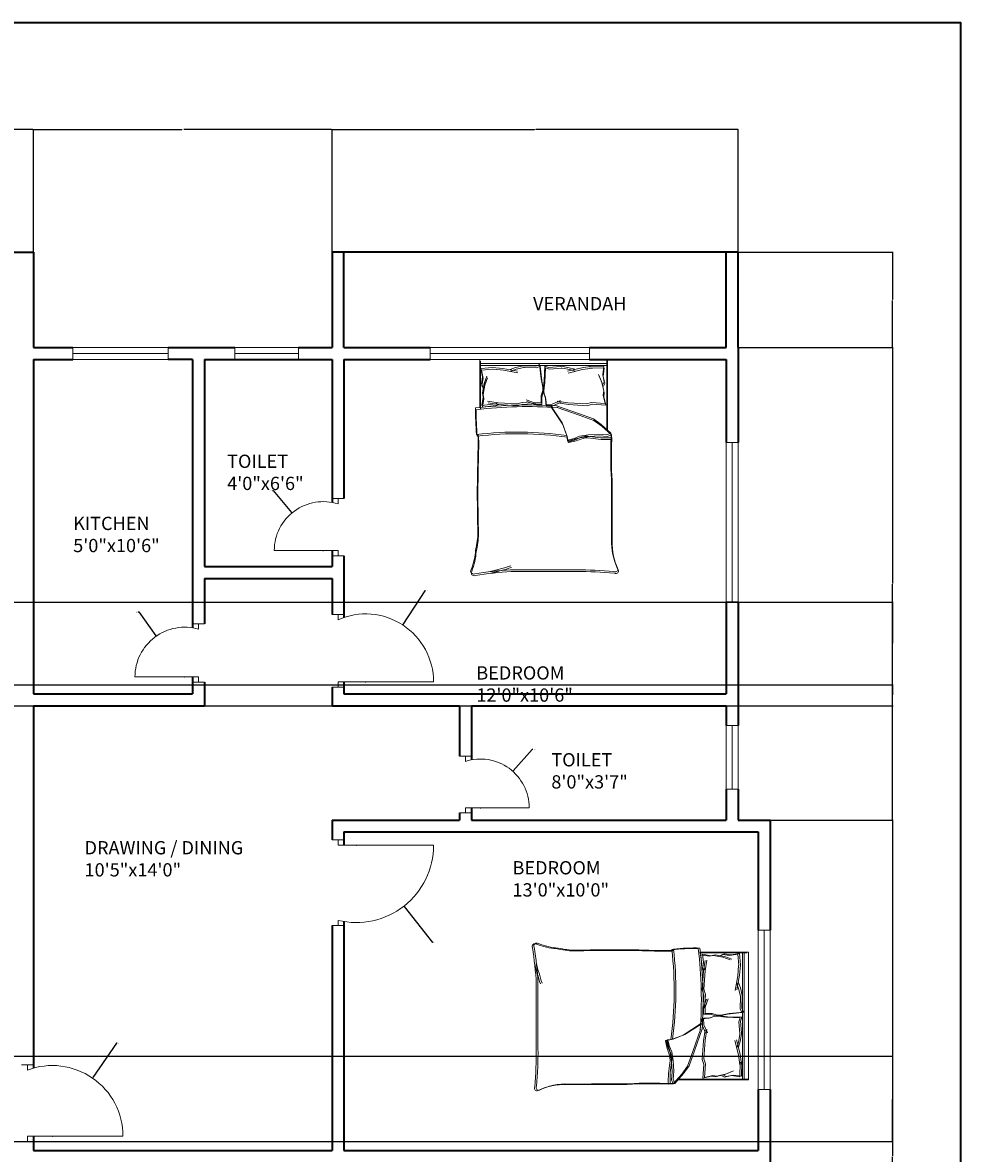
# Model space of a CAD drawing. Units: inches. Extents: x 1937 to 2996, y 1402 to 2323.
# Tile 10 of 10: x 2643 to 2996, y 1897 to 2323. Entities that reach past the tile are written whole.
import ezdxf

# ---------------------------------------------------------------- set-up
doc = ezdxf.new("R2010")
doc.units = ezdxf.units.IN
for name, color, linetype, lineweight in [('A-ANNO-DIMS', 2, 'Continuous', 18), ('A-ANNO-TTLB', 7, 'Continuous', 35), ('A-AREA-IDEN', 7, 'Continuous', 18), ('A-DOOR', 11, 'Continuous', 18), ('A-FURN', 8, 'Continuous', 13), ('A-GLAZ', 141, 'Continuous', 18), ('A-WALL', 7, 'Continuous', 35)]:
    doc.layers.add(name, color=color, linetype=linetype, lineweight=lineweight)
doc.styles.get("Standard").update_dxf_attribs({"font": 'arial.ttf'})
doc.dimstyles.get("Standard").update_dxf_attribs({"dimtxt": 0.18, "dimasz": 0.18, "dimexe": 0.18, "dimexo": 0.0625, "dimgap": 0.09, "dimtad": 0, "dimtih": 1, "dimtoh": 1, "dimdec": 4, "dimzin": 0, "dimdsep": 46, "dimtxsty": 'Standard', "dimcen": 0.09, "dimadec": 0, "dimazin": 0, "dimtfac": 1, "dimtdec": 4, "dimtofl": 0, "dimtmove": 0, "dimatfit": 3, "dimfxl": 1, "dimtolj": 1, "dimtzin": 0, "dimarcsym": 0})

# ---------------------------------------------------------------- blocks, each defined once
blk = doc.blocks.new('BED-DOUBLE')
for p, q in [((-24.01, -18.11), (-24.01, 0)), ((-24.01, -18.11), (-24.01, 0)), ((-24.01, 0), (24.01, 0)), ((23.78, 0), (23.78, -26.61)), ((23.78, 0), (23.78, -26.61)), ((24.01, 0), (24.01, -0.64)), ((-24.01, -1.53), (23.78, -1.53)), ((-24.01, -1.53), (23.78, -1.53)), ((-23.78, -18.75), (-23.78, -0.64)), ((-23.78, -18.75), (-23.78, -0.64)), ((-23.78, -2.17), (24.01, -2.17)), ((-23.78, -2.17), (24.01, -2.17)), ((-23.59, -3.34), (-19.3, -3.01)), ((-23.59, -3.34), (-19.31, -3.01)), ((-23.59, -3.32), (-23.01, -6.5)), ((-23.59, -3.32), (-23.01, -6.5)), ((-23.36, -3.98), (-19.08, -3.65)), ((-23.36, -3.98), (-19.08, -3.65)), ((-23.36, -3.96), (-22.78, -7.14)), ((-23.36, -3.96), (-22.78, -7.14)), ((-19.31, -3.01), (-19.2, -3.03)), ((-19.3, -3.01), (-19.2, -3.03)), ((-19.2, -3.03), (-15.38, -3.32)), ((-19.2, -3.03), (-15.38, -3.32)), ((-19.08, -3.65), (-18.97, -3.67)), ((-19.08, -3.65), (-18.97, -3.67)), ((-18.97, -3.67), (-15.15, -3.96)), ((-18.97, -3.67), (-15.15, -3.96)), ((-15.38, -3.32), (-9.88, -4.33)), ((-15.38, -3.32), (-9.88, -4.33)), ((-15.15, -3.96), (-9.65, -4.97)), ((-15.15, -3.96), (-9.65, -4.97)), ((-12.63, -3.75), (-10.61, -3.03)), ((-12.63, -3.75), (-10.61, -3.03)), ((-12.4, -4.39), (-10.38, -3.67)), ((-12.4, -4.39), (-10.38, -3.67)), ((-10.61, -3.03), (-7.71, -2.3)), ((-10.61, -3.03), (-7.71, -2.3)), ((-10.38, -3.67), (-7.49, -2.94)), ((-10.38, -3.67), (-7.49, -2.94)), ((-7.71, -2.3), (-7.39, -2.3)), ((-7.71, -2.3), (-7.39, -2.3)), ((-7.49, -2.94), (-7.16, -2.94)), ((-7.49, -2.94), (-7.16, -2.94)), ((-7.39, -2.3), (-2.95, -2.45)), ((-7.39, -2.3), (-2.95, -2.45)), ((-7.16, -2.94), (-2.72, -3.09)), ((-7.16, -2.94), (-2.72, -3.09)), ((-2.95, -2.45), (-1.5, -1.87)), ((-2.95, -2.45), (-1.5, -1.87)), ((-2.72, -3.09), (-1.27, -2.51)), ((-2.72, -3.09), (-1.27, -2.51)), ((-1.5, -1.87), (-0.92, -7.22)), ((-1.5, -1.87), (-0.92, -7.22)), ((-1.27, -2.51), (-0.7, -7.86)), ((-1.27, -2.51), (-0.7, -7.86)), ((0.49, -2.49), (0.25, -7.87)), ((0.49, -2.49), (0.25, -7.87)), ((0.72, -3.13), (0.48, -8.51)), ((0.72, -3.13), (0.48, -8.51)), ((1.97, -2.98), (0.49, -2.49)), ((1.97, -2.98), (0.49, -2.49)), ((2.2, -3.62), (0.72, -3.13)), ((2.2, -3.62), (0.72, -3.13)), ((6.4, -2.56), (1.97, -2.98)), ((6.4, -2.56), (1.97, -2.98)), ((6.63, -3.2), (2.2, -3.62)), ((6.63, -3.2), (2.2, -3.62)), ((6.72, -2.54), (6.4, -2.56)), ((6.72, -2.54), (6.4, -2.56)), ((6.95, -3.18), (6.63, -3.2)), ((6.95, -3.18), (6.63, -3.2)), ((9.65, -3.08), (6.72, -2.54)), ((9.65, -3.08), (6.72, -2.54)), ((9.88, -3.72), (6.95, -3.18)), ((9.88, -3.72), (6.95, -3.18)), ((14.43, -3.07), (9.01, -4.42)), ((14.43, -3.07), (9.01, -4.42)), ((14.66, -3.71), (9.24, -5.06)), ((14.66, -3.71), (9.24, -5.06)), ((11.72, -3.67), (9.65, -3.08)), ((11.72, -3.67), (9.65, -3.08)), ((11.94, -4.31), (9.88, -3.72)), ((11.94, -4.31), (9.88, -3.72)), ((18.23, -2.54), (14.43, -3.07)), ((18.23, -2.54), (14.43, -3.07)), ((18.46, -3.18), (14.66, -3.71)), ((18.46, -3.18), (14.66, -3.71)), ((22.63, -2.56), (17.23, -2.46)), ((17.23, -2.46), (18.23, -2.54)), ((22.63, -2.56), (17.23, -2.46)), ((17.23, -2.46), (18.23, -2.54)), ((22.86, -3.2), (17.45, -3.1)), ((17.45, -3.1), (18.46, -3.18)), ((22.86, -3.2), (17.45, -3.1)), ((17.45, -3.1), (18.46, -3.18)), ((22.63, -2.56), (22.25, -5.77)), ((22.63, -2.56), (22.25, -5.77)), ((22.86, -3.2), (22.48, -6.41)), ((22.86, -3.2), (22.48, -6.41)), ((24.01, -0.64), (24.01, -27.25)), ((24.01, -0.64), (24.01, -27.25)), ((-23.01, -6.5), (-23.45, -9.1)), ((-23.01, -6.5), (-23.45, -9.1)), ((-22.78, -7.14), (-23.22, -9.74)), ((-22.78, -7.14), (-23.22, -9.74)), ((-22.43, -8.96), (-21.42, -6.21)), ((-22.43, -8.96), (-21.42, -6.21)), ((-22.21, -9.59), (-21.19, -6.85)), ((-22.2, -9.59), (-21.19, -6.85)), ((-0.92, -7.22), (-0.35, -10.4)), ((-0.92, -7.22), (-0.35, -10.4)), ((-0.7, -7.86), (-0.12, -11.04)), ((-0.7, -7.86), (-0.12, -11.04)), ((0.25, -7.87), (-0.13, -11.08)), ((0.25, -7.87), (-0.13, -11.08)), ((0.48, -8.51), (0.1, -11.72)), ((0.48, -8.51), (0.1, -11.72)), ((21.83, -8.26), (20.64, -5.58)), ((21.82, -8.26), (20.64, -5.58)), ((22.05, -8.9), (20.87, -6.22)), ((22.05, -8.9), (20.87, -6.22)), ((22.63, -11.83), (21.82, -8.26)), ((22.63, -11.83), (21.83, -8.26)), ((22.25, -5.77), (22.84, -8.34)), ((22.25, -5.77), (22.84, -8.34)), ((22.84, -8.34), (22.33, -9.38)), ((22.84, -8.34), (22.33, -9.38)), ((22.48, -6.41), (23.07, -8.98)), ((22.48, -6.41), (23.07, -8.98)), ((-23.45, -9.1), (-22.87, -10.11)), ((-23.45, -9.1), (-22.87, -10.11)), ((-23.22, -9.74), (-22.64, -10.75)), ((-23.22, -9.74), (-22.64, -10.75)), ((-23.01, -12.57), (-22.43, -8.96)), ((-23.01, -12.57), (-22.43, -8.96)), ((-22.72, -14.16), (-23.01, -12.57)), ((-22.72, -14.16), (-23.01, -12.57)), ((-22.78, -13.21), (-22.2, -9.59)), ((-22.78, -13.21), (-22.21, -9.59)), ((-0.35, -11.7), (-0.92, -13.58)), ((-0.35, -11.7), (-0.92, -13.58)), ((-0.12, -12.34), (-0.7, -14.22)), ((-0.12, -12.34), (-0.7, -14.22)), ((-0.35, -10.4), (-0.35, -11.7)), ((-0.35, -10.4), (-0.35, -11.7)), ((-0.13, -11.08), (-0.05, -12.38)), ((-0.13, -11.08), (-0.05, -12.38)), ((-0.12, -11.04), (-0.12, -12.34)), ((-0.12, -11.04), (-0.12, -12.34)), ((-0.05, -12.38), (0.65, -14.22)), ((-0.05, -12.38), (0.65, -14.22)), ((0.1, -11.72), (0.18, -13.02)), ((0.1, -11.72), (0.18, -13.02)), ((22.86, -12.47), (22.05, -8.9)), ((22.86, -12.47), (22.05, -8.9)), ((22.44, -13.43), (22.63, -11.83)), ((22.44, -13.43), (22.63, -11.83)), ((23.07, -8.98), (22.56, -10.02)), ((23.07, -8.98), (22.56, -10.02)), ((22.67, -14.07), (22.86, -12.47)), ((22.67, -14.07), (22.86, -12.47)), ((-23.3, -17.34), (-22.72, -14.16)), ((-23.3, -17.34), (-22.72, -14.16)), ((-18.2, -16.62), (-23.3, -17.34)), ((-18.2, -16.62), (-23.3, -17.34)), ((-23.07, -17.98), (-22.49, -14.8)), ((-23.07, -17.98), (-22.49, -14.8)), ((-22.49, -14.8), (-22.78, -13.21)), ((-22.49, -14.8), (-22.78, -13.21)), ((-21.1, -15.63), (-17.07, -16.3)), ((-21.1, -15.63), (-17.07, -16.3)), ((-20.87, -16.27), (-16.84, -16.93)), ((-20.87, -16.27), (-16.84, -16.93)), ((-17.07, -16.3), (-18.2, -16.62)), ((-17.07, -16.3), (-18.2, -16.62)), ((-16.84, -16.93), (-17.98, -17.26)), ((-16.84, -16.93), (-17.98, -17.26)), ((-17.07, -16.3), (-10.06, -16.73)), ((-17.07, -16.3), (-10.06, -16.73)), ((-16.84, -16.93), (-9.83, -17.37)), ((-16.84, -16.93), (-9.83, -17.37)), ((-10.06, -16.73), (-8.1, -16.17)), ((-10.06, -16.73), (-8.1, -16.17)), ((-9.83, -17.37), (-7.87, -16.81)), ((-9.83, -17.37), (-7.87, -16.81)), ((-8.1, -16.17), (-2.97, -16.57)), ((-8.1, -16.17), (-2.97, -16.57)), ((-7.87, -16.81), (-2.74, -17.21)), ((-7.87, -16.81), (-2.74, -17.21)), ((-3.38, -16.26), (-6.53, -15.17)), ((-3.38, -16.26), (-6.53, -15.17)), ((-3.15, -16.9), (-6.3, -15.81)), ((-3.15, -16.9), (-6.3, -15.81)), ((-0.92, -16.26), (-3.38, -16.26)), ((-0.92, -16.26), (-3.38, -16.26)), ((-0.7, -16.9), (-3.15, -16.9)), ((-0.7, -16.9), (-3.15, -16.9)), ((-0.92, -13.58), (-0.92, -16.26)), ((-0.92, -13.58), (-0.92, -16.26)), ((-0.7, -14.22), (-0.7, -16.9)), ((-0.7, -14.22), (-0.7, -16.9)), ((0.18, -13.02), (0.87, -14.86)), ((0.18, -13.02), (0.87, -14.86)), ((0.65, -14.22), (0.81, -16.89)), ((0.65, -14.22), (0.81, -16.89)), ((0.81, -16.89), (3.27, -16.74)), ((0.81, -16.89), (3.27, -16.74)), ((0.87, -14.86), (1.04, -17.53)), ((0.87, -14.86), (1.04, -17.53)), ((3.27, -16.74), (6.34, -15.45)), ((3.27, -16.74), (6.34, -15.45)), ((3.49, -17.38), (6.56, -16.09)), ((3.49, -17.38), (6.56, -16.09)), ((5.08, -15.63), (9.11, -16.3)), ((5.08, -15.63), (9.11, -16.3)), ((5.31, -16.27), (9.34, -16.93)), ((5.31, -16.27), (9.34, -16.93)), ((9.11, -16.3), (16.12, -16.73)), ((9.11, -16.3), (16.12, -16.73)), ((9.34, -16.93), (16.35, -17.37)), ((9.34, -16.93), (16.35, -17.37)), ((16.12, -16.73), (18.08, -16.17)), ((16.12, -16.73), (18.08, -16.17)), ((16.35, -17.37), (18.31, -16.81)), ((16.35, -17.37), (18.31, -16.81)), ((18.08, -16.17), (23.21, -16.57)), ((18.08, -16.17), (23.21, -16.57)), ((18.31, -16.81), (23.44, -17.21)), ((18.31, -16.81), (23.44, -17.21)), ((23.21, -16.57), (22.44, -13.43)), ((23.21, -16.57), (22.44, -13.43)), ((23.44, -17.21), (22.67, -14.07)), ((23.44, -17.21), (22.67, -14.07)), ((-17.98, -17.26), (-23.07, -17.98)), ((-17.98, -17.26), (-23.07, -17.98)), ((1.04, -17.53), (3.49, -17.38)), ((1.04, -17.53), (3.49, -17.38)), ((2.77, -17.38), (6.97, -23.88)), ((2.77, -17.38), (6.96, -23.88)), ((3, -18.02), (7.19, -24.52)), ((3, -18.02), (7.19, -24.52)), ((13.16, -20.32), (4.82, -17.38)), ((13.16, -20.32), (4.82, -17.38)), ((13.39, -20.96), (5.05, -18.02)), ((13.39, -20.96), (5.05, -18.02)), ((18.74, -22.33), (13.16, -20.32)), ((18.74, -22.33), (13.16, -20.32)), ((18.96, -22.97), (13.39, -20.96)), ((18.96, -22.97), (13.39, -20.96)), ((6.96, -23.88), (8.67, -28.37)), ((6.97, -23.88), (8.67, -28.37)), ((7.19, -24.52), (8.9, -29)), ((7.19, -24.52), (8.9, -29)), ((21.68, -24.5), (18.74, -22.33)), ((21.68, -24.5), (18.74, -22.33)), ((21.91, -25.13), (18.96, -22.97)), ((21.91, -25.13), (18.96, -22.97)), ((25.38, -27.75), (21.68, -24.5)), ((25.38, -27.75), (21.68, -24.5)), ((25.61, -28.39), (21.91, -25.13)), ((25.61, -28.39), (21.91, -25.13)), ((8.67, -28.37), (8.98, -30.38)), ((8.67, -28.37), (8.98, -30.38)), ((8.9, -29), (9.21, -31.02)), ((8.9, -29), (9.21, -31.02)), ((8.98, -30.38), (11.46, -29.76)), ((8.98, -30.38), (11.46, -29.76)), ((11.46, -29.76), (13.47, -28.83)), ((11.46, -29.76), (13.47, -28.83)), ((11.68, -30.4), (13.7, -29.47)), ((11.68, -30.4), (13.7, -29.47)), ((13.47, -28.83), (16.88, -28.37)), ((13.47, -28.83), (16.88, -28.37)), ((13.7, -29.47), (17.11, -29)), ((13.7, -29.47), (17.1, -29)), ((16.88, -28.37), (20.75, -28.06)), ((16.88, -28.37), (20.75, -28.06)), ((17.1, -29), (20.98, -28.69)), ((17.11, -29), (20.98, -28.69)), ((20.75, -28.06), (23.85, -28.37)), ((20.75, -28.06), (23.85, -28.37)), ((20.98, -28.69), (24.07, -29)), ((20.98, -28.69), (24.07, -29)), ((23.85, -28.37), (25.38, -27.75)), ((23.85, -28.37), (25.38, -27.75)), ((24.07, -29), (25.61, -28.39)), ((24.07, -29), (25.61, -28.39)), ((25.46, -29.49), (25.38, -27.75, 3.87)), ((25.46, -29.49), (25.38, -27.75, 3.87)), ((25.69, -30.13), (25.61, -28.39, 3.87)), ((25.69, -30.13), (25.61, -28.39, 3.87)), ((9.21, -31.02), (11.68, -30.4)), ((9.21, -31.02), (11.68, -30.4)), ((-12.42, -79.25), (12.19, -79.25)), ((-12.42, -79.25), (12.19, -79.25)), ((-12.19, -79.88), (12.42, -79.88)), ((-12.19, -79.88), (12.42, -79.88))]:
    blk.add_line(p, q)
for centre, radius, start, end in [((57.68, -20.1), 83.31, 178.7218, 185.604), ((57.68, -20.1), 83.31, 178.7218, 185.604), ((-6.13, -182.05), 164.97, 86.0865, 96.7821), ((-6.13, -182.05), 164.97, 86.0865, 96.7821), ((57.91, -20.74), 83.31, 178.7218, 185.604), ((57.91, -20.74), 83.31, 178.7218, 185.604), ((-5.9, -182.69), 164.97, 86.0865, 96.7821), ((-5.9, -182.69), 164.97, 86.0865, 96.7821), ((-9.73, -156.32), 129.02, 81.7845, 96.9006), ((-9.73, -156.32), 129.02, 81.7845, 96.9006), ((-9.5, -156.96), 129.02, 81.7845, 96.9006), ((-9.5, -156.96), 129.02, 81.7845, 96.9006), ((-194.79, -31.17), 170.11, 358.4762, 1.0082), ((-194.79, -31.17), 170.11, 358.4762, 1.0082), ((-194.56, -31.81), 170.11, 358.4762, 1.0082), ((-194.56, -31.81), 170.11, 358.4762, 1.0082), ((3.67, -1.48), 29.65, 280.6617, 289.8806), ((3.67, -1.48), 29.65, 280.6617, 289.8806), ((16.26, -35.07), 6.22, 78.6608, 113.7384), ((16.26, -35.07), 6.22, 78.6608, 113.7384), ((16.49, -35.71), 6.22, 78.6608, 113.7384), ((16.49, -35.71), 6.22, 78.6608, 113.7384), ((23.84, 6.66), 36.18, 259.8763, 272.5657), ((23.84, 6.66), 36.18, 259.8763, 272.5657), ((24.07, 6.02), 36.18, 259.8763, 272.5657), ((24.07, 6.02), 36.18, 259.8763, 272.5657), ((154.78, -36.32), 129.5, 176.9791, 183.8365), ((154.78, -36.32), 129.5, 176.9791, 183.8365), ((9.15, -30.44), 0.185, 160.2464, 271.1377), ((9.15, -30.44), 0.185, 160.2464, 271.1377), ((9.38, -31.08), 0.185, 160.2464, 271.1377), ((9.38, -31.08), 0.185, 160.2464, 271.1377), ((3.9, -2.12), 29.65, 280.6617, 289.8806), ((3.9, -2.12), 29.65, 280.6617, 289.8806), ((155.01, -36.95), 129.5, 176.9791, 183.8365), ((155.01, -36.95), 129.5, 176.9791, 183.8365), ((457.34, -50.61), 482.31, 178.2277, 181.7185), ((457.34, -50.61), 482.31, 178.2277, 181.7185), ((457.57, -51.25), 482.31, 178.2277, 181.7185), ((457.57, -51.25), 482.31, 178.2277, 181.7185), ((-4536.23, -67.82), 4561.86, 0.00217, 0.28689), ((-4536.23, -67.82), 4561.86, 0.00217, 0.28689), ((-4536, -68.46), 4561.86, 0.00217, 0.28689), ((-4536, -68.46), 4561.86, 0.00217, 0.28689), ((-54.38, -64.52), 29.63, 346.0648, 358.9113), ((-54.38, -64.52), 29.63, 346.0648, 358.9113), ((-54.16, -65.15), 29.63, 346.0648, 358.9113), ((-54.16, -65.15), 29.63, 346.0648, 358.9113), ((48.67, -68.67), 23.07, 177.4714, 206.4681), ((48.67, -68.67), 23.07, 177.4714, 206.4681), ((-49.14, -70.28), 23.56, 337.9751, 356.652), ((-49.14, -70.28), 23.56, 337.9751, 356.652), ((-48.92, -70.91), 23.56, 337.9751, 356.652), ((-48.92, -70.91), 23.56, 337.9751, 356.652), ((48.9, -69.31), 23.07, 177.4714, 206.4681), ((48.9, -69.31), 23.07, 177.4714, 206.4681), ((-26.4, -79.72), 1.09, 146.1736, 293.4781), ((-26.4, -79.72), 1.09, 146.1736, 293.4781), ((-26.17, -80.36), 1.09, 146.1736, 293.4781), ((-26.17, -80.36), 1.09, 146.1736, 293.4781), ((-6.06, -200.84), 121.76, 92.9958, 99.4091), ((-6.06, -200.84), 121.76, 92.9958, 99.4091), ((-5.83, -201.48), 121.76, 92.9958, 99.4091), ((-5.83, -201.48), 121.76, 92.9958, 99.4091), ((-44.71, 23.71), 106.46, 283.3832, 287.7053), ((-44.71, 23.71), 106.46, 283.3832, 287.7053), ((-44.48, 23.07), 106.46, 283.3832, 287.7053), ((-44.48, 23.07), 106.46, 283.3832, 287.7053), ((13.67, -212.28), 133.04, 84.4998, 90.6351), ((13.67, -212.28), 133.04, 84.4998, 90.6351), ((13.9, -212.92), 133.04, 84.4998, 90.6351), ((13.9, -212.92), 133.04, 84.4998, 90.6351), ((26.93, -78.87), 1.1, 242.6588, 356.02), ((26.93, -78.87), 1.1, 242.6588, 356.02), ((27.15, -79.51), 1.1, 242.6588, 356.02), ((27.15, -79.51), 1.1, 242.6588, 356.02)]:
    blk.add_arc(centre, radius, start, end)
blk = doc.blocks.new('WINDOW-60IN')
for p, q in [((0, 2.25), (0, -2.25)), ((0, 2.25), (60, 2.25)), ((0, -2.25), (0, 0)), ((0, 0), (60, 0)), ((60, 0), (60, 2.25)), ((60, 2.25), (60, -2.25)), ((60, -2.25), (0, -2.25))]:
    blk.add_line(p, q)
blk = doc.blocks.new('WINDOW-60IN-JAMB-B')
for p, q in [((2.25, 60), (-2.25, 60)), ((-2.25, 60), (-2.25, 0)), ((0, 0), (0, 60)), ((0, 60), (2.25, 60)), ((2.25, 0), (2.25, 60)), ((-2.25, 0), (2.25, 0)), ((2.25, 0), (0, 0))]:
    blk.add_line(p, q)
blk = doc.blocks.new('WINDOW-24IN-JAMB-B')
for p, q in [((0, -2.25), (0, 2.25)), ((0, 2.25), (0, 0)), ((24, 2.25), (0, 2.25)), ((0, 0), (24, 0)), ((24, 0), (24, 2.25)), ((24, 2.25), (24, -2.25)), ((0, -2.25), (24, -2.25))]:
    blk.add_line(p, q)
blk = doc.blocks.new('*D29')
at = {"layer": 'A-ANNO-DIMS', "color": 0, "lineweight": -2, "transparency": 16777216}
for p, q in [((2517.65, 2236.87), (2517.65, 2283.14)), ((2517.83, 2282.96), (2581.87, 2282.96)), ((2646.47, 2282.96), (2582.43, 2282.96)), ((2646.65, 2236.87), (2646.65, 2283.14))]:
    blk.add_line(p, q, dxfattribs=at)
at = {"layer": 'A-ANNO-DIMS', "color": 0, "transparency": 16777216}
for points in [[(2517.83, 2282.99), (2517.83, 2282.93), (2517.65, 2282.96)], [(2646.47, 2282.99), (2646.47, 2282.93), (2646.65, 2282.96)]]:
    blk.add_solid(points, dxfattribs=at)
at = {"layer": 'Defpoints', "color": 0, "transparency": 16777216}
for p in [(2646.65, 2282.96), (2517.65, 2236.81), (2646.65, 2236.81)]:
    blk.add_point(p, dxfattribs=at)
at = {"layer": 'A-ANNO-DIMS', "color": 0, "transparency": 16777216, "insert": (2582.15, 2282.96), "char_height": 0.18, "attachment_point": 5}
blk.add_mtext('\\A1;129', dxfattribs=at)
blk = doc.blocks.new('*D30')
at = {"layer": 'A-ANNO-DIMS', "color": 0, "lineweight": -2, "transparency": 16777216}
for p, q in [((2646.65, 2236.87), (2646.65, 2283.14)), ((2646.83, 2282.96), (2702.51, 2282.96)), ((2758.97, 2282.96), (2703.28, 2282.96)), ((2759.15, 2236.87), (2759.15, 2283.14))]:
    blk.add_line(p, q, dxfattribs=at)
at = {"layer": 'A-ANNO-DIMS', "color": 0, "transparency": 16777216}
for points in [[(2646.83, 2282.99), (2646.83, 2282.93), (2646.65, 2282.96)], [(2758.97, 2282.99), (2758.97, 2282.93), (2759.15, 2282.96)]]:
    blk.add_solid(points, dxfattribs=at)
at = {"layer": 'Defpoints', "color": 0, "transparency": 16777216}
for p in [(2759.15, 2282.96), (2646.65, 2236.81), (2759.15, 2236.81)]:
    blk.add_point(p, dxfattribs=at)
at = {"layer": 'A-ANNO-DIMS', "color": 0, "transparency": 16777216, "insert": (2702.9, 2282.96), "char_height": 0.18, "attachment_point": 5}
blk.add_mtext('\\A1;112.5', dxfattribs=at)
blk = doc.blocks.new('*D31')
at = {"layer": 'A-ANNO-DIMS', "color": 0, "lineweight": -2, "transparency": 16777216}
for p, q in [((2759.15, 2236.87), (2759.15, 2283.14)), ((2759.33, 2282.96), (2835.37, 2282.96)), ((2911.97, 2282.96), (2835.93, 2282.96)), ((2912.15, 2236.87), (2912.15, 2283.14))]:
    blk.add_line(p, q, dxfattribs=at)
at = {"layer": 'A-ANNO-DIMS', "color": 0, "transparency": 16777216}
for points in [[(2759.33, 2282.99), (2759.33, 2282.93), (2759.15, 2282.96)], [(2911.97, 2282.99), (2911.97, 2282.93), (2912.15, 2282.96)]]:
    blk.add_solid(points, dxfattribs=at)
at = {"layer": 'Defpoints', "color": 0, "transparency": 16777216}
for p in [(2912.15, 2282.96), (2759.15, 2236.81), (2912.15, 2236.81)]:
    blk.add_point(p, dxfattribs=at)
at = {"layer": 'A-ANNO-DIMS', "color": 0, "transparency": 16777216, "insert": (2835.65, 2282.96), "char_height": 0.18, "attachment_point": 5}
blk.add_mtext('\\A1;153', dxfattribs=at)
blk = doc.blocks.new('*D41')
at = {"layer": 'A-ANNO-DIMS', "color": 0, "lineweight": -2, "transparency": 16777216}
for p, q in [((2924.21, 2022.81), (2970.48, 2022.81)), ((2970.3, 2022.63), (2970.3, 1896.24)), ((2970.3, 1769.49), (2970.3, 1895.87)), ((2924.21, 1769.31), (2970.48, 1769.31))]:
    blk.add_line(p, q, dxfattribs=at)
at = {"layer": 'A-ANNO-DIMS', "color": 0, "transparency": 16777216}
for points in [[(2970.27, 2022.63), (2970.33, 2022.63), (2970.3, 2022.81)], [(2970.27, 1769.49), (2970.33, 1769.49), (2970.3, 1769.31)]]:
    blk.add_solid(points, dxfattribs=at)
at = {"layer": 'Defpoints', "color": 0, "transparency": 16777216}
for p in [(2924.15, 2022.81), (2970.3, 2022.81), (2924.15, 1769.31)]:
    blk.add_point(p, dxfattribs=at)
at = {"layer": 'A-ANNO-DIMS', "color": 0, "transparency": 16777216, "insert": (2970.3, 1896.06), "char_height": 0.18, "attachment_point": 5}
blk.add_mtext('\\A1;253.5', dxfattribs=at)
blk = doc.blocks.new('*D42')
at = {"layer": 'A-ANNO-DIMS', "color": 0, "lineweight": -2, "transparency": 16777216}
for p, q in [((2912.21, 2200.81), (2970.48, 2200.81)), ((2970.3, 2200.63), (2970.3, 2111.99)), ((2970.3, 2022.99), (2970.3, 2111.62)), ((2912.21, 2022.81), (2970.48, 2022.81))]:
    blk.add_line(p, q, dxfattribs=at)
at = {"layer": 'A-ANNO-DIMS', "color": 0, "transparency": 16777216}
for points in [[(2970.27, 2200.63), (2970.33, 2200.63), (2970.3, 2200.81)], [(2970.27, 2022.99), (2970.33, 2022.99), (2970.3, 2022.81)]]:
    blk.add_solid(points, dxfattribs=at)
at = {"layer": 'Defpoints', "color": 0, "transparency": 16777216}
for p in [(2912.15, 2200.81), (2970.3, 2200.81), (2912.15, 2022.81)]:
    blk.add_point(p, dxfattribs=at)
at = {"layer": 'A-ANNO-DIMS', "color": 0, "transparency": 16777216, "insert": (2970.3, 2111.81), "char_height": 0.18, "attachment_point": 5}
blk.add_mtext('\\A1;178', dxfattribs=at)
blk = doc.blocks.new('*D43')
at = {"layer": 'A-ANNO-DIMS', "color": 0, "lineweight": -2, "transparency": 16777216}
for p, q in [((2912.21, 2236.81), (2970.48, 2236.81)), ((2970.3, 2236.63), (2970.3, 2218.99)), ((2970.3, 2200.99), (2970.3, 2218.62)), ((2912.21, 2200.81), (2970.48, 2200.81))]:
    blk.add_line(p, q, dxfattribs=at)
at = {"layer": 'A-ANNO-DIMS', "color": 0, "transparency": 16777216}
for points in [[(2970.27, 2236.63), (2970.33, 2236.63), (2970.3, 2236.81)], [(2970.27, 2200.99), (2970.33, 2200.99), (2970.3, 2200.81)]]:
    blk.add_solid(points, dxfattribs=at)
at = {"layer": 'Defpoints', "color": 0, "transparency": 16777216}
for p in [(2912.15, 2236.81), (2970.3, 2236.81), (2912.15, 2200.81)]:
    blk.add_point(p, dxfattribs=at)
at = {"layer": 'A-ANNO-DIMS', "color": 0, "transparency": 16777216, "insert": (2970.3, 2218.81), "char_height": 0.18, "attachment_point": 5}
blk.add_mtext('\\A1;36', dxfattribs=at)
blk = doc.blocks.new('*D50')
at = {"layer": 'A-ANNO-DIMS', "color": 0, "lineweight": -2, "transparency": 16777216}
for p, q in [((2292.71, 1933.76), (2970.48, 1933.76)), ((2970.3, 1933.58), (2970.3, 1917.9)), ((2970.3, 1901.85), (2970.3, 1917.53)), ((2292.71, 1901.67), (2970.48, 1901.67))]:
    blk.add_line(p, q, dxfattribs=at)
at = {"layer": 'A-ANNO-DIMS', "color": 0, "transparency": 16777216}
for points in [[(2970.27, 1933.58), (2970.33, 1933.58), (2970.3, 1933.76)], [(2970.27, 1901.85), (2970.33, 1901.85), (2970.3, 1901.67)]]:
    blk.add_solid(points, dxfattribs=at)
at = {"layer": 'Defpoints', "color": 0, "transparency": 16777216}
for p in [(2292.65, 1933.76), (2970.3, 1933.76), (2292.65, 1901.67)]:
    blk.add_point(p, dxfattribs=at)
at = {"layer": 'A-ANNO-DIMS', "color": 0, "transparency": 16777216, "insert": (2970.3, 1917.71), "char_height": 0.18, "attachment_point": 5}
blk.add_mtext('\\A1;32.085', dxfattribs=at)
blk = doc.blocks.new('*D51')
at = {"layer": 'A-ANNO-DIMS', "color": 0, "lineweight": -2, "transparency": 16777216}
for p, q in [((2175.71, 2073.74), (2970.48, 2073.74)), ((2970.3, 2073.56), (2970.3, 2069.95)), ((2970.3, 2065.99), (2970.3, 2069.59)), ((2175.71, 2065.81), (2970.48, 2065.81))]:
    blk.add_line(p, q, dxfattribs=at)
at = {"layer": 'A-ANNO-DIMS', "color": 0, "transparency": 16777216}
for points in [[(2970.27, 2073.56), (2970.33, 2073.56), (2970.3, 2073.74)], [(2970.27, 2065.99), (2970.33, 2065.99), (2970.3, 2065.81)]]:
    blk.add_solid(points, dxfattribs=at)
at = {"layer": 'Defpoints', "color": 0, "transparency": 16777216}
for p in [(2175.65, 2073.74), (2970.3, 2073.74), (2175.65, 2065.81)]:
    blk.add_point(p, dxfattribs=at)
at = {"layer": 'A-ANNO-DIMS', "color": 0, "transparency": 16777216, "insert": (2970.3, 2069.77), "char_height": 0.18, "attachment_point": 5}
blk.add_mtext('\\A1;7.931', dxfattribs=at)
blk = doc.blocks.new('*D52')
at = {"layer": 'A-ANNO-DIMS', "color": 0, "lineweight": -2, "transparency": 16777216}
for p, q in [((2175.71, 2104.94), (2970.48, 2104.94)), ((2970.3, 2104.76), (2970.3, 2089.52)), ((2970.3, 2073.92), (2970.3, 2089.16)), ((2175.71, 2073.74), (2970.48, 2073.74))]:
    blk.add_line(p, q, dxfattribs=at)
at = {"layer": 'A-ANNO-DIMS', "color": 0, "transparency": 16777216}
for points in [[(2970.27, 2104.76), (2970.33, 2104.76), (2970.3, 2104.94)], [(2970.27, 2073.92), (2970.33, 2073.92), (2970.3, 2073.74)]]:
    blk.add_solid(points, dxfattribs=at)
at = {"layer": 'Defpoints', "color": 0, "transparency": 16777216}
for p in [(2175.65, 2104.94), (2970.3, 2104.94), (2175.65, 2073.74)]:
    blk.add_point(p, dxfattribs=at)
at = {"layer": 'A-ANNO-DIMS', "color": 0, "transparency": 16777216, "insert": (2970.3, 2089.34), "char_height": 0.18, "attachment_point": 5}
blk.add_mtext('\\A1;31.204', dxfattribs=at)
blk = doc.blocks.new('*D61')
at = {"layer": 'A-ANNO-DIMS', "color": 0, "lineweight": -2, "transparency": 16777216}
for p, q in [((2768.19, 2013.29), (2768.37, 2013.29)), ((2768.28, 2013.2), (2768.28, 2013.38)), ((2797.07, 1976.66), (2786.38, 1990.26)), ((2797.25, 1976.66), (2797.07, 1976.66))]:
    blk.add_line(p, q, dxfattribs=at)
at = {"layer": 'A-ANNO-DIMS', "color": 0, "transparency": 16777216}
blk.add_solid([(2786.41, 1990.28), (2786.36, 1990.24), (2786.27, 1990.4)], dxfattribs=at)
at = {"layer": 'Defpoints', "color": 0, "transparency": 16777216}
for p in [(2768.28, 2013.29), (2786.27, 1990.4)]:
    blk.add_point(p, dxfattribs=at)
at = {"layer": 'A-ANNO-DIMS', "color": 0, "transparency": 16777216, "insert": (2797.73, 1976.66), "char_height": 0.18, "attachment_point": 5}
blk.add_mtext('\\A1;R29.12', dxfattribs=at)
blk = doc.blocks.new('*D70')
at = {"layer": 'A-ANNO-DIMS', "color": 0, "lineweight": -2, "transparency": 16777216}
for p, q in [((2677.99, 1938.7), (2669.02, 1925.73)), ((2678.17, 1938.7), (2677.99, 1938.7)), ((2653.72, 1903.7), (2653.9, 1903.7)), ((2653.81, 1903.61), (2653.81, 1903.79))]:
    blk.add_line(p, q, dxfattribs=at)
at = {"layer": 'A-ANNO-DIMS', "color": 0, "transparency": 16777216}
blk.add_solid([(2669, 1925.74), (2669.05, 1925.71), (2668.92, 1925.58)], dxfattribs=at)
at = {"layer": 'Defpoints', "color": 0, "transparency": 16777216}
for p in [(2668.92, 1925.58), (2653.81, 1903.7)]:
    blk.add_point(p, dxfattribs=at)
at = {"layer": 'A-ANNO-DIMS', "color": 0, "transparency": 16777216, "insert": (2678.65, 1938.7), "char_height": 0.18, "attachment_point": 5}
blk.add_mtext('\\A1;R26.59', dxfattribs=at)
blk = doc.blocks.new('*D72')
at = {"layer": 'A-ANNO-DIMS', "color": 0, "lineweight": -2, "transparency": 16777216}
for p, q in [((2794.14, 2109.2), (2785.85, 2096.46)), ((2794.32, 2109.2), (2794.14, 2109.2)), ((2771.68, 2074.84), (2771.86, 2074.84)), ((2771.77, 2074.75), (2771.77, 2074.93))]:
    blk.add_line(p, q, dxfattribs=at)
at = {"layer": 'A-ANNO-DIMS', "color": 0, "transparency": 16777216}
blk.add_solid([(2785.82, 2096.48), (2785.87, 2096.45), (2785.75, 2096.31)], dxfattribs=at)
at = {"layer": 'Defpoints', "color": 0, "transparency": 16777216}
for p in [(2785.75, 2096.31), (2771.77, 2074.84)]:
    blk.add_point(p, dxfattribs=at)
at = {"layer": 'A-ANNO-DIMS', "color": 0, "transparency": 16777216, "insert": (2794.87, 2109.2), "char_height": 0.18, "attachment_point": 5}
blk.add_mtext('\\A1;R25.624', dxfattribs=at)
blk = doc.blocks.new('*D78')
at = {"layer": 'A-ANNO-DIMS', "color": 0, "lineweight": -2, "transparency": 16777216}
for p, q in [((2736.75, 2146.99), (2736.93, 2146.99)), ((2736.93, 2146.99), (2743.89, 2138.65)), ((2755.71, 2124.38), (2755.89, 2124.38)), ((2755.8, 2124.29), (2755.8, 2124.47))]:
    blk.add_line(p, q, dxfattribs=at)
at = {"layer": 'A-ANNO-DIMS', "color": 0, "transparency": 16777216}
blk.add_solid([(2743.92, 2138.67), (2743.87, 2138.63), (2744.01, 2138.51)], dxfattribs=at)
at = {"layer": 'Defpoints', "color": 0, "transparency": 16777216}
for p in [(2744.01, 2138.51), (2755.8, 2124.38)]:
    blk.add_point(p, dxfattribs=at)
at = {"layer": 'A-ANNO-DIMS', "color": 0, "transparency": 16777216, "insert": (2736.2, 2146.99), "char_height": 0.18, "attachment_point": 5}
blk.add_mtext('\\A1;R18.404', dxfattribs=at)
blk = doc.blocks.new('*D79')
at = {"layer": 'A-ANNO-DIMS', "color": 0, "lineweight": -2, "transparency": 16777216}
for p, q in [((2686.15, 2101.2), (2686.33, 2101.2)), ((2686.33, 2101.2), (2692.72, 2092.16)), ((2703.56, 2076.7), (2703.74, 2076.7)), ((2703.65, 2076.61), (2703.65, 2076.79))]:
    blk.add_line(p, q, dxfattribs=at)
at = {"layer": 'A-ANNO-DIMS', "color": 0, "transparency": 16777216}
blk.add_solid([(2692.75, 2092.18), (2692.7, 2092.14), (2692.83, 2092.02)], dxfattribs=at)
at = {"layer": 'Defpoints', "color": 0, "transparency": 16777216}
for p in [(2692.83, 2092.02), (2703.65, 2076.7)]:
    blk.add_point(p, dxfattribs=at)
at = {"layer": 'A-ANNO-DIMS', "color": 0, "transparency": 16777216, "insert": (2685.6, 2101.2), "char_height": 0.18, "attachment_point": 5}
blk.add_mtext('\\A1;R18.756', dxfattribs=at)
blk = doc.blocks.new('*D80')
at = {"layer": 'A-ANNO-DIMS', "color": 0, "lineweight": -2, "transparency": 16777216}
for p, q in [((2834.56, 2049.37), (2827.37, 2041.29)), ((2834.74, 2049.37), (2834.56, 2049.37)), ((2814.97, 2027.45), (2815.15, 2027.45)), ((2815.06, 2027.36), (2815.06, 2027.54))]:
    blk.add_line(p, q, dxfattribs=at)
at = {"layer": 'A-ANNO-DIMS', "color": 0, "transparency": 16777216}
blk.add_solid([(2827.35, 2041.31), (2827.39, 2041.27), (2827.25, 2041.15)], dxfattribs=at)
at = {"layer": 'Defpoints', "color": 0, "transparency": 16777216}
for p in [(2827.25, 2041.15), (2815.06, 2027.45)]:
    blk.add_point(p, dxfattribs=at)
at = {"layer": 'A-ANNO-DIMS', "color": 0, "transparency": 16777216, "insert": (2835.29, 2049.37), "char_height": 0.18, "attachment_point": 5}
blk.add_mtext('\\A1;R18.336', dxfattribs=at)

msp = doc.modelspace()

# ---------------------------------------------------------------- linework, layer by layer
at = {"layer": 'A-ANNO-TTLB'}
msp.add_lwpolyline([(1937.1125, 2323.2883), (2995.8132, 2323.2883), (2995.8132, 1401.6335), (1937.1125, 1401.6335)], close=True, dxfattribs=at)
at = {"layer": 'A-DOOR'}
for p, q in [((2759.1473, 2143.9134), (2763.6473, 2143.9134)), ((2763.6473, 2143.9134), (2761.3973, 2143.9134)), ((2761.3973, 2143.9134), (2761.3973, 2141.9134)), ((2761.3973, 2124.3812), (2737.3973, 2124.3812)), ((2759.1473, 2122.3812), (2763.6473, 2122.3812)), ((2761.3973, 2122.3812), (2761.3973, 2124.3812)), ((2763.6473, 2122.3812), (2761.3973, 2122.3812)), ((2706.6473, 2096.7087), (2711.1473, 2096.7087)), ((2711.1473, 2096.7087), (2708.8973, 2096.7087)), ((2708.8973, 2096.7087), (2708.8973, 2094.7087)), ((2763.6473, 2100.2666), (2759.1473, 2100.2666)), ((2759.1473, 2100.2666), (2761.3973, 2100.2666)), ((2761.3973, 2100.2666), (2761.3973, 2098.2666)), ((2708.8973, 2076.7002), (2684.8973, 2076.7002)), ((2708.8973, 2074.7002), (2708.8973, 2076.7002)), ((2706.6473, 2074.7002), (2711.1473, 2074.7002)), ((2711.1473, 2074.7002), (2708.8973, 2074.7002)), ((2763.6473, 2072.8373), (2759.1473, 2072.8373)), ((2759.1473, 2072.8373), (2761.3973, 2072.8373)), ((2761.3973, 2072.8373), (2761.3973, 2074.8373)), ((2761.3973, 2074.8373), (2797.3973, 2074.8373)), ((2807.1473, 2046.8934), (2811.6473, 2046.8934)), ((2811.6473, 2046.8934), (2809.3973, 2046.8934)), ((2809.3973, 2046.8934), (2809.3973, 2044.8934)), ((2807.1473, 2025.4548), (2811.6473, 2025.4548)), ((2809.3973, 2025.4548), (2809.3973, 2027.4548)), ((2809.3973, 2027.4548), (2833.3973, 2027.4548)), ((2811.6473, 2025.4548), (2809.3973, 2025.4548)), ((2763.6473, 2015.2946), (2759.1473, 2015.2946)), ((2759.1473, 2015.2946), (2760.5703, 2015.2946)), ((2760.5703, 2015.2946), (2761.3973, 2015.2946)), ((2761.3973, 2015.2946), (2761.3973, 2013.2946)), ((2761.3973, 2013.2946), (2797.3973, 2013.2946)), ((2759.1473, 1982.9988), (2763.6473, 1982.9988)), ((2761.3973, 1982.9988), (2761.3973, 1984.9988)), ((2763.6473, 1982.9988), (2761.3973, 1982.9988)), ((2642.1473, 1930.5712), (2646.6473, 1930.5712)), ((2646.6473, 1930.5712), (2644.3973, 1930.5712)), ((2644.3973, 1930.5712), (2644.3973, 1928.5712)), ((2646.6473, 1901.7001), (2642.1473, 1901.7001)), ((2642.1473, 1901.7001), (2644.3973, 1901.7001)), ((2644.3973, 1901.7001), (2644.3973, 1903.7001)), ((2644.3973, 1903.7001), (2680.3973, 1903.7001))]:
    msp.add_line(p, q, dxfattribs=at)
for centre, radius, start, end in [((2755.801, 2124.3812), 18.4037, 72.296643, 180), ((2771.7732, 2074.8373), 25.6241, 360, 113.886693), ((2703.6537, 2076.7002), 18.7564, 73.765781, 180), ((2815.0618, 2027.4548), 18.3355, 0, 107.995057), ((2768.2772, 2013.2946), 29.1201, 256.334222, 360), ((2653.806, 1903.7001), 26.5913, 360, 110.721567)]:
    msp.add_arc(centre, radius, start, end, dxfattribs=at)
at = {"layer": 'A-GLAZ'}
for p, q in [((2661.4638, 2200.8061), (2661.4638, 2196.3061)), ((2661.4638, 2200.8061), (2698.9521, 2200.8061)), ((2697.4638, 2198.5561), (2697.4638, 2200.8061)), ((2697.4638, 2200.8061), (2697.4638, 2198.5561)), ((2661.4638, 2196.3061), (2661.4638, 2198.5561)), ((2661.4638, 2198.5561), (2697.4638, 2198.5561)), ((2661.4638, 2196.3061), (2697.4638, 2196.3061)), ((2697.4638, 2196.3061), (2697.4638, 2198.5561)), ((2909.8973, 2058.4632), (2907.6473, 2058.4632)), ((2907.6473, 2058.4632), (2912.1473, 2058.4632)), ((2907.6473, 2058.4632), (2907.6473, 2033.1971)), ((2909.8973, 2034.4632), (2909.8973, 2058.4632)), ((2912.1473, 2034.4632), (2912.1473, 2058.4632)), ((2907.6473, 2034.4632), (2912.1473, 2034.4632)), ((2912.1473, 2034.4632), (2909.8973, 2034.4632))]:
    msp.add_line(p, q, dxfattribs=at)
at = {"layer": 'A-WALL'}
for p, q in [((2612.1965, 2236.8061), (2646.6473, 2236.8061)), ((2646.6473, 2236.8061), (2646.6473, 2200.8061)), ((2912.1473, 2236.8061), (2759.1473, 2236.8061)), ((2759.1473, 2236.8061), (2759.1473, 2200.8061)), ((2763.6473, 2200.8061), (2763.6473, 2236.8061)), ((2907.6473, 2200.8061), (2907.6473, 2236.8061)), ((2912.1473, 2200.8061), (2912.1473, 2236.8061)), ((2646.6473, 2200.8061), (2661.4638, 2200.8061)), ((2697.4638, 2200.8061), (2722.5061, 2200.8061)), ((2746.5061, 2200.8061), (2759.1473, 2200.8061)), ((2763.6473, 2200.8061), (2796.0587, 2200.8061)), ((2856.0587, 2200.8061), (2907.6473, 2200.8061)), ((2912.1473, 2200.8061), (2912.1473, 2165.0312)), ((2646.6473, 2196.3061), (2646.6473, 2070.3061)), ((2646.6473, 2196.3061), (2661.4638, 2196.3061)), ((2706.6473, 2196.3061), (2697.4638, 2196.3061)), ((2706.6473, 2196.3061), (2706.6473, 2095.2162)), ((2711.1473, 2196.3061), (2711.1473, 2118.3061)), ((2711.1473, 2196.3061), (2746.5061, 2196.3061)), ((2746.5061, 2196.3061), (2759.1473, 2196.3061)), ((2759.1473, 2196.3061), (2759.1473, 2142.4781)), ((2763.6473, 2196.3061), (2763.6473, 2143.9134)), ((2763.6473, 2196.3061), (2796.0587, 2196.3061)), ((2856.0587, 2196.3061), (2907.6473, 2196.3061)), ((2907.6473, 2196.3061), (2907.6473, 2165.0312)), ((2759.1473, 2124.3812), (2759.1473, 2118.3061)), ((2763.6473, 2122.3812), (2763.6473, 2099.1387)), ((2711.1473, 2118.3061), (2759.1473, 2118.3061)), ((2711.1473, 2113.8061), (2759.1473, 2113.8061)), ((2711.1473, 2113.8061), (2711.1473, 2096.7087)), ((2759.1473, 2113.8061), (2759.1473, 2100.2666)), ((2907.6473, 2105.0312), (2907.6473, 2070.3061)), ((2912.1473, 2105.0312), (2912.1473, 2058.4632)), ((2706.6473, 2076.7002), (2706.6473, 2070.3061)), ((2711.1473, 2074.7002), (2711.1473, 2065.8061)), ((2759.1473, 2072.8373), (2759.1473, 2065.8061)), ((2763.6473, 2074.8373), (2763.6473, 2070.3061)), ((2646.6473, 2070.3061), (2706.6473, 2070.3061)), ((2763.6473, 2070.3061), (2907.6473, 2070.3061)), ((2646.6473, 2065.8061), (2711.1473, 2065.8061)), ((2646.6473, 2065.8061), (2646.6473, 1929.3097)), ((2759.1473, 2065.8061), (2807.1473, 2065.8061)), ((2807.1473, 2065.8061), (2807.1473, 2046.8934)), ((2811.6473, 2065.8061), (2811.6473, 2045.4696)), ((2811.6473, 2065.8061), (2907.6473, 2065.8061)), ((2907.6473, 2065.8061), (2907.6473, 2058.4632)), ((2907.6473, 2034.4632), (2907.6473, 2022.8061)), ((2912.1473, 2034.4632), (2912.1473, 2022.8061)), ((2807.1473, 2025.4548), (2807.1473, 2022.8061)), ((2811.6473, 2027.4548), (2811.6473, 2022.8061)), ((2759.1473, 2022.8061), (2807.1473, 2022.8061)), ((2759.1473, 2022.8061), (2759.1473, 2015.2946)), ((2811.6473, 2022.8061), (2907.6473, 2022.8061)), ((2912.1473, 2022.8061), (2924.1473, 2022.8061)), ((2924.1473, 2022.8061), (2924.1473, 1981.2943)), ((2763.6473, 2018.3061), (2919.6473, 2018.3061)), ((2763.6473, 2018.3061), (2763.6473, 2013.2946)), ((2919.6473, 2018.3061), (2919.6473, 1981.2943)), ((2759.1473, 1982.9988), (2759.1473, 1898.3061)), ((2763.6473, 1984.5448), (2763.6473, 1898.3061)), ((2919.6473, 1921.2943), (2919.6473, 1898.3061)), ((2924.1473, 1921.2943), (2924.1473, 1898.3061)), ((2646.6473, 1903.7001), (2646.6473, 1898.3061)), ((2646.6473, 1898.3061), (2759.1473, 1898.3061)), ((2763.6473, 1898.3061), (2919.6473, 1898.3061)), ((2924.1473, 1898.3061), (2924.1473, 1860.2229))]:
    msp.add_line(p, q, dxfattribs=at)

# ---------------------------------------------------------------- block references
at = {"layer": 'A-FURN'}
msp.add_blockref('BED-DOUBLE', (2838.835, 2196.3061), dxfattribs=at)
at = {"layer": 'A-FURN', "rotation": 269.9999998331858}
msp.add_blockref('BED-DOUBLE', (2915.9652, 1948.9492), dxfattribs=at)
at = {"layer": 'A-GLAZ'}
msp.add_blockref('WINDOW-24IN-JAMB-B', (2722.5061, 2198.5561), dxfattribs=at)
at = {"layer": 'A-GLAZ', "extrusion": (0, 0, -1), "zscale": -1, "rotation": 90}
msp.add_blockref('WINDOW-60IN-JAMB-B', (-2796.0587, 2198.5561), dxfattribs=at)
at = {"layer": 'A-GLAZ', "rotation": 90}
for p in [(2909.8973, 2105.0312), (2921.8973, 1921.2943)]:
    msp.add_blockref('WINDOW-60IN', p, dxfattribs=at)

# ---------------------------------------------------------------- texts
at = {"layer": 'A-AREA-IDEN', "char_height": 5, "attachment_point": 1}
for s, width, insert in [('VERANDAH', 137.071433, (2834.8728, 2219.8875)), ('TOILET\\P4\'0"x6\'6"', 92.658771, (2719.6403, 2160.4841)), ('KITCHEN\\P5\'0"x10\'6"', 138.230625, (2661.65, 2137.0764)), ('BEDROOM\\P12\'0"x10\'6"', 112.516786, (2813.4895, 2080.7262)), ('TOILET\\P8\'0"x3\'7"', 92.130948, (2841.7468, 2048.0042)), ('DRAWING / DINING \\P10\'5"x14\'0"', 162.39206, (2665.9299, 2014.8617)), ('BEDROOM\\P13\'0"x10\'0"', 126.813526, (2827.1182, 2007.3111))]:
    msp.add_mtext_dynamic_manual_height_columns(s, width=width, gutter_width=12.5, heights=[0], dxfattribs=dict(at, insert=insert))

# ---------------------------------------------------------------- dimensions: what is measured, and where the dimension line sits
at = {"layer": 'A-ANNO-DIMS'}
for base, p1, p2, override, picture, middle in [((2646.6473, 2282.9561), (2517.6473, 2236.8061), (2646.6473, 2236.8061), {"dimdec": 0, "dimlfac": 1, "dimrnd": 0, "dimzin": 0, "dimdsep": 46, "dimlunit": 2}, '*D29', (2582.1473, 2282.9561)), ((2759.1473, 2282.9561), (2646.6473, 2236.8061), (2759.1473, 2236.8061), {"dimdec": 1, "dimlfac": 1, "dimrnd": 0, "dimzin": 0, "dimdsep": 46, "dimlunit": 2}, '*D30', (2702.8973, 2282.9561)), ((2912.1473, 2282.9561), (2759.1473, 2236.8061), (2912.1473, 2236.8061), {"dimdec": 0, "dimlfac": 1, "dimrnd": 0, "dimzin": 0, "dimdsep": 46, "dimlunit": 2}, '*D31', (2835.6473, 2282.9561))]:
    dim = msp.add_linear_dim(base=base, p1=p1, p2=p2, dimstyle='Standard', override=override, dxfattribs=at)
    dim.commit()
    dim.dimension.update_dxf_attribs({"geometry": picture, "text_midpoint": middle})
for base, p1, p2, override, picture, middle in [((2970.2973, 2236.8061), (2912.1473, 2200.8061), (2912.1473, 2236.8061), {"dimdec": 0, "dimlfac": 1, "dimrnd": 0, "dimzin": 0, "dimdsep": 46, "dimlunit": 2}, '*D43', (2970.2973, 2218.8061)), ((2970.2973, 2200.8061), (2912.1473, 2022.8061), (2912.1473, 2200.8061), {"dimdec": 0, "dimlfac": 1, "dimrnd": 0, "dimzin": 0, "dimdsep": 46, "dimlunit": 2}, '*D42', (2970.2973, 2111.8061)), ((2970.2973, 2104.9416), (2175.6473, 2073.7376), (2175.6473, 2104.9416), {"dimdec": 3, "dimlfac": 1, "dimrnd": 0, "dimzin": 0, "dimdsep": 46, "dimlunit": 2}, '*D52', (2970.2973, 2089.3396)), ((2970.29731, 2073.73761), (2175.64731, 2065.80612), (2175.64731, 2073.73761), {"dimdec": 3, "dimlfac": 1, "dimrnd": 0, "dimzin": 0, "dimdsep": 46, "dimlunit": 2}, '*D51', (2970.29731, 2069.77186)), ((2970.2973, 2022.8061), (2924.1473, 1769.3061), (2924.1473, 2022.8061), {"dimdec": 1, "dimlfac": 1, "dimrnd": 0, "dimzin": 0, "dimdsep": 46, "dimlunit": 2}, '*D41', (2970.2973, 1896.0561)), ((2970.2973, 1933.7562), (2292.6473, 1901.671), (2292.6473, 1933.7562), {"dimdec": 3, "dimlfac": 1, "dimrnd": 0, "dimzin": 0, "dimdsep": 46, "dimlunit": 2}, '*D50', (2970.2973, 1917.7136))]:
    dim = msp.add_linear_dim(base=base, p1=p1, p2=p2, angle=90, dimstyle='Standard', override=override, dxfattribs=at)
    dim.commit()
    dim.dimension.update_dxf_attribs({"geometry": picture, "text_midpoint": middle})
for center, mpoint, override, picture, middle in [((2755.801, 2124.3812), (2744.0086, 2138.5104), {"dimdec": 3, "dimlfac": 1, "dimrnd": 0, "dimzin": 0, "dimdsep": 46, "dimlunit": 2}, '*D78', (2736.2038, 2146.988)), ((2771.7732, 2074.8373), (2785.7499, 2096.3139), {"dimdec": 3, "dimlfac": 1, "dimrnd": 0, "dimzin": 0, "dimdsep": 46, "dimlunit": 2}, '*D72', (2794.8653, 2109.1999)), ((2703.6537, 2076.7002), (2692.8255, 2092.0153), {"dimdec": 3, "dimlfac": 1, "dimrnd": 0, "dimzin": 0, "dimdsep": 46, "dimlunit": 2}, '*D79', (2685.5989, 2101.2044)), ((2815.06179, 2027.45478), (2827.24805, 2041.15465), {"dimdec": 3, "dimlfac": 1, "dimrnd": 0, "dimzin": 0, "dimdsep": 46, "dimlunit": 2}, '*D80', (2835.2895, 2049.37457)), ((2768.2772, 2013.2946), (2786.2721, 1990.3999), {"dimdec": 2, "dimlfac": 1, "dimrnd": 0, "dimzin": 0, "dimdsep": 46, "dimlunit": 2}, '*D61', (2797.7279, 1976.6631)), ((2653.806, 1903.7001), (2668.9209, 1925.5779), {"dimdec": 2, "dimlfac": 1, "dimrnd": 0, "dimzin": 0, "dimdsep": 46, "dimlunit": 2}, '*D70', (2678.6499, 1938.7045))]:
    dim = msp.add_radius_dim(center=center, mpoint=mpoint, dimstyle='Standard', override=override, dxfattribs=at)
    dim.commit()
    dim.dimension.update_dxf_attribs({"geometry": picture, "text_midpoint": middle, "dimtype": 164})

doc.saveas('drawing.dxf')
